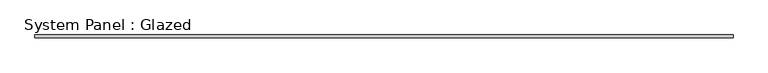
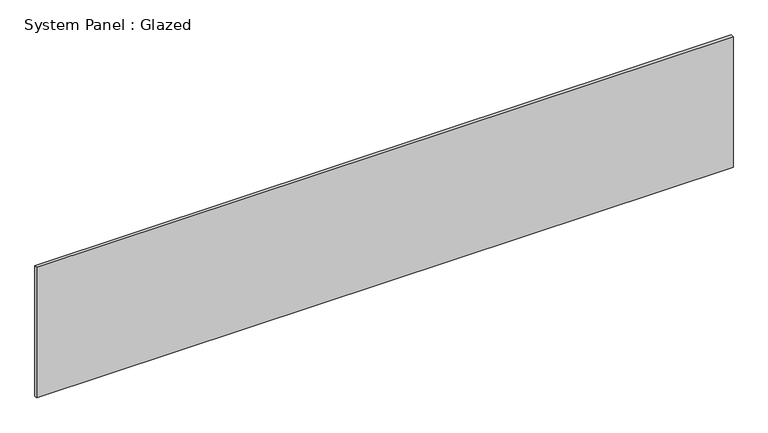
"""IFC4 building model written with IfcOpenShell, lengths in millimetres: plate geometry, System Panel : Glazed."""

from ifc_helpers import new_model, si_unit, origin, origin_with_axes, place, context, project, spatial, polyline, outline, extrude, source, transform, mapped, element, save


def system_panel_glazed_fe04ab03(model_context):
    return source(origin(), model_context, "Body", "SweptSolid", [
        extrude(outline(polyline([(3076.575, 19.05), (-3076.575, 19.05), (-3076.575, 44.45), (3076.575, 44.45), (3076.575, 19.05)])), origin_with_axes(), (0.0, 0.0, 1.0), 1219.2),
    ])


if __name__ == "__main__":
    model = new_model("IFC4")
    model_context = context("Model", 3, world=origin())
    ifc_project = project(units=[si_unit("LENGTHUNIT", "METRE", prefix="MILLI")], contexts=[model_context])
    site = spatial("IfcSite", under=ifc_project)
    building = spatial("IfcBuilding", under=site)
    placement = place(None, origin())
    system_panel_glazed_shape = system_panel_glazed_fe04ab03(model_context)
    element("IfcPlate", 1, ObjectType="System Panel : Glazed", at=placement, inside=building, context=model_context, shape_type="MappedRepresentation", body=[
        mapped(system_panel_glazed_shape, transform((0.0, 0.0, 0.0), x_axis=(1.0, 0.0, 0.0), y_axis=(0.0, 1.0, 0.0), z_axis=(0.0, 0.0, 1.0))),
    ])
    save(model, "model.ifc")

# Revit data of these elements
# Type "System Panel : Glazed"
#   Construction Type Id = "GSP4R"
#   Analytic Construction = "1/8 in Pilkington single glazing"
#   Visual Light Transmittance = 0.9
#   Solar Heat Gain Coefficient = 0.86
#   Heat Transfer Coefficient (U) = 1.18115 BTU/(h·ft²·°F)
# Element 1 (IfcPlate, "System Panel : Glazed")
#   Materials on its faces: "Glass"
# Materials
#   "Glass": class "Glass", colour RGB 0 128 192, transparency 0.75, Description = "Soda Lime Glass", Cost = 0
